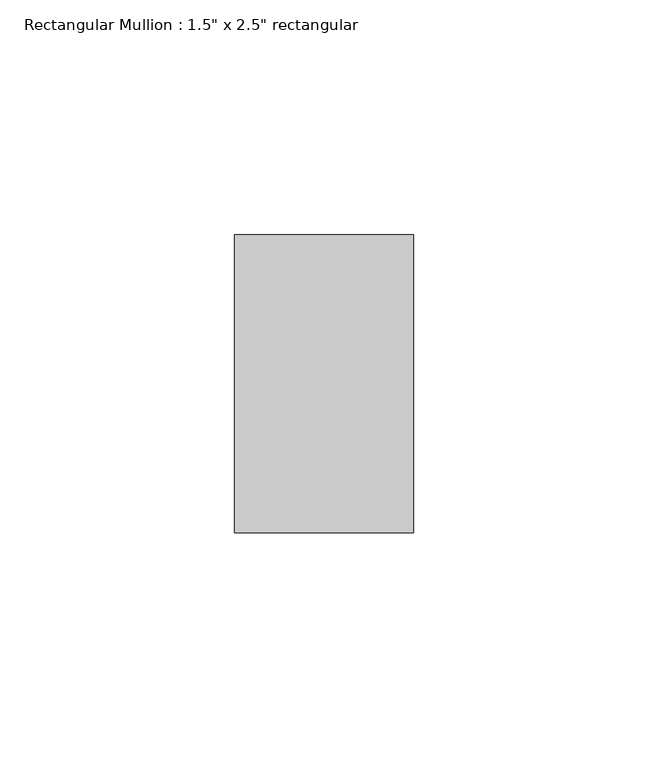
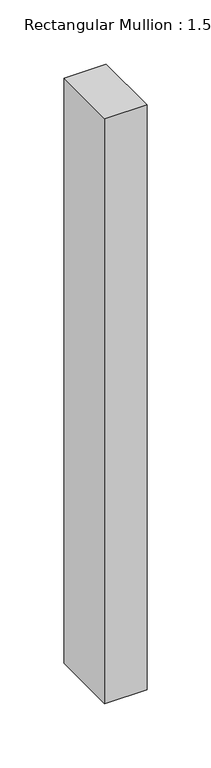
"""IFC4 building model written with IfcOpenShell, lengths in millimetres: member geometry."""

from ifc_helpers import new_model, si_unit, frame, origin, place, context, project, spatial, polyline, outline, extrude, source, transform, mapped, element, save


def member_acd33549(model_context):
    return source(origin(), model_context, "Body", "SweptSolid", [
        extrude(outline(polyline([(0.0, 31.75), (0.0, -31.75), (-38.1, -31.75), (-38.1, 31.75), (0.0, 31.75)])), frame((0.0, 0.0, -557.1903046), z_axis=(0.0, 0.0, 1.0), x_axis=(1.0, 0.0, 0.0)), (0.0, 0.0, 1.0), 557.1903046),
    ])


if __name__ == "__main__":
    model = new_model("IFC4")
    model_context = context("Model", 3, world=origin())
    ifc_project = project(units=[si_unit("LENGTHUNIT", "METRE", prefix="MILLI")], contexts=[model_context])
    site = spatial("IfcSite", under=ifc_project)
    building = spatial("IfcBuilding", under=site)
    placement = place(None, origin())
    member_shape = member_acd33549(model_context)
    element("IfcMember", 1, ObjectType="Rectangular Mullion : 1.5\" x 2.5\" rectangular", at=placement, inside=building, context=model_context, shape_type="MappedRepresentation", body=[
        mapped(member_shape, transform((0.0, 0.0, 0.0), x_axis=(1.0, 0.0, 0.0), y_axis=(0.0, 1.0, 0.0), z_axis=(0.0, 0.0, 1.0))),
    ])
    save(model, "model.ifc")

# Revit data of these elements
# Type "Rectangular Mullion : 1.5\" x 2.5\" rectangular"
#   built-in parameter 1007304 = 0.208333 (stored number, unit not read)
#   built-in parameter 1007301 = 0.0625 (stored number, unit not read)
#   built-in parameter 1007300 = 0.0625 (stored number, unit not read)
# Element 1 (IfcMember, "Rectangular Mullion : 1.5\" x 2.5\" rectangular")
#   Materials on its faces: "Leather - Black"
# Materials
#   "Leather - Black": class "Generic", colour RGB 40 40 40, transparency 0, Cost = 0
